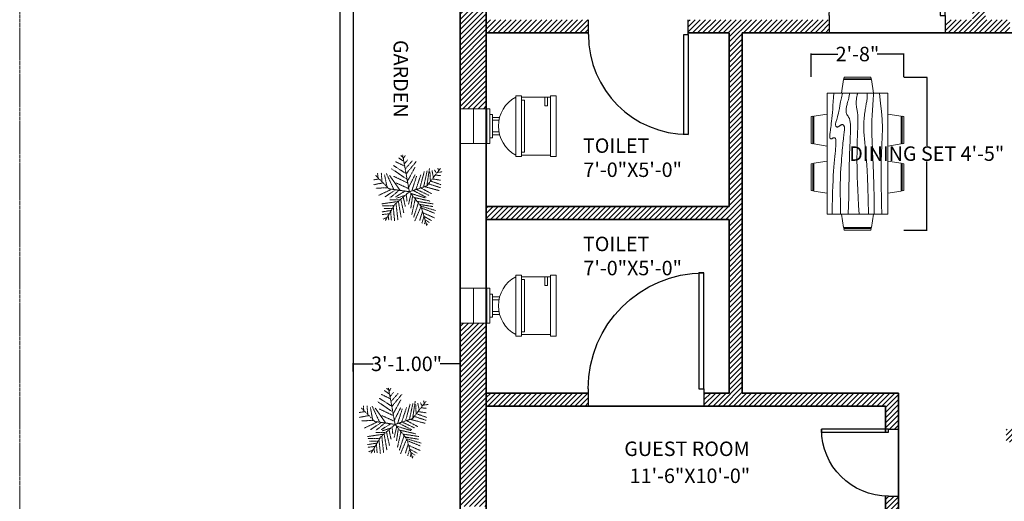
# Model space of a CAD drawing. Units: inches. Extents: x 2202345 to 2203065, y -970921 to -970107.
# Tile 3 of 5: x 2202345 to 2202685, y -970515 to -970348. Entities that reach past the tile are written whole.
import ezdxf

# ---------------------------------------------------------------- set-up
doc = ezdxf.new("R2010")
doc.units = ezdxf.units.IN
doc.header["$MEASUREMENT"] = 0
doc.linetypes.add('HIDDEN', pattern=[0.375, 0.25, -0.125])
doc.layers.get('0').update_dxf_attribs({"color": 13})
for name, color, linetype, lineweight in [('A-ANNO-DIMS', 2, 'Continuous', 18), ('A-ANNO-TTLB', 7, 'HIDDEN', 18), ('A-AREA-IDEN', 7, 'Continuous', 18), ('A-WALL-PATT', 8, 'Continuous', 13), ('C-PROP', 7, 'Continuous', 25), ('doors', 252, 'Continuous', 25), ('furniture', 250, 'Continuous', 18), ('garden', 114, 'HIDDEN', 13), ('PLUMBING FIXTURES', 8, 'Continuous', 18), ('walls', 252, 'Continuous', 35), ('windows', 173, 'Continuous', 18)]:
    doc.layers.add(name, color=color, linetype=linetype, lineweight=lineweight)
doc.styles.get("Standard").update_dxf_attribs({"font": 'arial.ttf'})
doc.dimstyles.get("Standard").update_dxf_attribs({"dimtxt": 5, "dimasz": 0.18, "dimexe": 0.18, "dimexo": 0.0625, "dimgap": 0.09, "dimtad": 0, "dimtih": 1, "dimtoh": 1, "dimzin": 0, "dimdsep": 46, "dimlunit": 3, "dimtxsty": 'Standard', "dimcen": 0.09, "dimadec": 0, "dimazin": 0, "dimtfac": 1, "dimtofl": 0, "dimtmove": 0, "dimatfit": 3, "dimfxl": 1, "dimtolj": 1, "dimtzin": 0, "dimarcsym": 0})
pattern_1 = [(45, (0, 0), (-0.8838834765, 0.8838834765), [])]

# ---------------------------------------------------------------- blocks, each defined once
blk = doc.blocks.new('Dining Set - 36 x 72 in.')
for p, q in [((-22.2343, 26.00059), (-23.4847, 17.99762)), ((-22.2304, 26), (-5.7608, 26)), ((-22, 27.5), (-22.1562, 26.50042)), ((-5.8416, 26.5), (-22.1534, 26.5)), ((-22, 27.5), (-6, 27.5)), ((-5.8437, 26.49966), (-6, 27.5)), ((-4.5152, 17.99762), (-5.7655, 25.99926)), ((5.7657, 26.00059), (4.5153, 17.99762)), ((5.7696, 26), (22.2392, 26)), ((6, 27.5), (5.8438, 26.50042)), ((22.1584, 26.5), (5.8466, 26.5)), ((6, 27.5), (22, 27.5)), ((22.1563, 26.49966), (22, 27.5)), ((23.4848, 17.99762), (22.2345, 25.99926)), ((36, 18), (-36, 18)), ((-36, 18), (-36, -18)), ((36, -18), (36, 18)), ((-45.5, 8), (-44.5004, 8.15617)), ((-45.5, 8), (-45.5, -8)), ((-44.5, -8.15843), (-44.5, 8.15338)), ((-44.0006, 8.23428), (-35.9976, 9.48474)), ((-44, 8.23041), (-44, -8.23915)), ((44.0006, 8.23428), (35.9976, 9.48474)), ((44, 8.23041), (44, -8.23915)), ((44.5, -8.15843), (44.5, 8.15338)), ((45.5, 8), (44.5005, 8.15617)), ((45.5, 8), (45.5, -8)), ((-44.4997, -8.15631), (-45.5, -8)), ((-35.9976, -9.48476), (-43.9993, -8.2345)), ((35.9976, -9.48476), (43.9993, -8.2345)), ((44.4997, -8.15631), (45.5, -8)), ((-36, -18), (36, -18)), ((-22.2343, -26.0006), (-23.4847, -17.99762)), ((-4.5152, -17.99762), (-5.7655, -25.99928)), ((5.7657, -26.0006), (4.5153, -17.99762)), ((23.4848, -17.99762), (22.2345, -25.99928)), ((-22.2304, -26), (-5.7608, -26)), ((-22, -27.5), (-22.1562, -26.50044)), ((-5.8416, -26.5), (-22.1534, -26.5)), ((-22, -27.5), (-6, -27.5)), ((-5.8437, -26.49967), (-6, -27.5)), ((5.7696, -26), (22.2392, -26)), ((6, -27.5), (5.8438, -26.50044)), ((22.1584, -26.5), (5.8466, -26.5)), ((6, -27.5), (22, -27.5)), ((22.1563, -26.49967), (22, -27.5))]:
    blk.add_line(p, q)
for points in [[(-36, 15), (-31.1772, 14.97754), (-26.8079, 14.91406), (-22.8538, 14.81543), (-19.276, 14.6875), (-16.0362, 14.53613), (-13.0957, 14.36718), (-10.4159, 14.18652), (-7.9583, 14), (-5.6904, 13.81315), (-3.6035, 13.63021), (-1.6954, 13.45508), (0.0365, 13.29166), (1.5945, 13.14388), (2.9811, 13.01562), (4.1988, 12.9108), (5.25, 12.83333), (6.1393, 12.78613), (6.8802, 12.76823), (7.4883, 12.77767), (7.9792, 12.8125), (8.3685, 12.87077), (8.6719, 12.95052), (8.9049, 13.0498), (9.0833, 13.16666), (9.2205, 13.29899), (9.3216, 13.44401), (9.3895, 13.59879), (9.4271, 13.76041), (9.4373, 13.92594), (9.4232, 14.09245), (9.3875, 14.257), (9.3333, 14.41666), (9.2638, 14.56917), (9.1836, 14.71484), (9.0975, 14.85465), (9.0104, 14.98958), (8.9272, 15.1206), (8.8529, 15.2487), (8.7922, 15.37483), (8.75, 15.5), (8.7305, 15.62467), (8.7344, 15.74739), (8.7617, 15.86621), (8.8125, 15.97916), (8.8867, 16.08431), (8.9844, 16.17968), (9.1055, 16.26334), (9.25, 16.33333), (9.4189, 16.38802), (9.6172, 16.42708), (9.8506, 16.45052), (10.125, 16.45833), (10.4463, 16.45052), (10.8203, 16.42708), (11.2529, 16.38802), (11.75, 16.33333), (12.3184, 16.26318), (12.9694, 16.17838), (13.7151, 16.07991), (14.5677, 15.96875), (15.5395, 15.84586), (16.6426, 15.71224), (17.8893, 15.56884), (19.2917, 15.41666), (20.859, 15.25667), (22.5879, 15.08984), (24.4721, 14.91715), (26.5052, 14.73958), (28.6809, 14.5581), (30.9929, 14.3737), (33.4347, 14.18733), (36, 14)], [(-36, 10), (-28.9766, 10.14274), (-23.1725, 10.20442), (-18.4241, 10.19775), (-14.5677, 10.13541), (-11.4399, 10.03011), (-8.877, 9.89453), (-6.7154, 9.74137), (-4.7917, 9.58333), (-2.9698, 9.43082), (-1.2246, 9.28515), (0.4415, 9.14534), (2.026, 9.01041), (3.5266, 8.87939), (4.9408, 8.7513), (6.266, 8.62516), (7.5, 8.5), (8.6411, 8.37549), (9.6914, 8.2539), (10.6538, 8.13818), (11.5312, 8.03125), (12.3267, 7.93603), (13.043, 7.85547), (13.6831, 7.79248), (14.25, 7.75), (14.7471, 7.7303), (15.1797, 7.73307), (15.5537, 7.75732), (15.875, 7.80208), (16.1494, 7.86637), (16.3828, 7.94922), (16.5811, 8.04964), (16.75, 8.16666), (16.8944, 8.29915), (17.0143, 8.44531), (17.1089, 8.60319), (17.1771, 8.77083), (17.218, 8.94629), (17.2305, 9.1276), (17.2137, 9.31282), (17.1667, 9.5), (17.0895, 9.6875), (16.987, 9.875), (16.8649, 10.0625), (16.7292, 10.25), (16.5856, 10.4375), (16.4401, 10.625), (16.2985, 10.8125), (16.1667, 11), (16.05, 11.18733), (15.9518, 11.3737), (15.8752, 11.5581), (15.8229, 11.73958), (15.798, 11.91715), (15.8034, 12.08984), (15.842, 12.25667), (15.9167, 12.41666), (16.0295, 12.56836), (16.1784, 12.70833), (16.3605, 12.83268), (16.5729, 12.9375), (16.8127, 13.01888), (17.0768, 13.07291), (17.3625, 13.0957), (17.6667, 13.08333), (17.9894, 13.03312), (18.3418, 12.94726), (18.7382, 12.82918), (19.1927, 12.68229), (19.7195, 12.51001), (20.3327, 12.31575), (21.0465, 12.10294), (21.875, 11.875), (22.8357, 11.63354), (23.959, 11.37304), (25.2786, 11.08618), (26.8282, 10.76562), (28.6414, 10.40405), (30.752, 9.99414), (33.1936, 9.52856), (36, 9)], [(-36, 5.5), (-30.7157, 5.3348), (-26.069, 5.20963), (-21.9946, 5.11767), (-18.4271, 5.05208), (-15.3009, 5.00602), (-12.5508, 4.97265), (-10.1112, 4.94515), (-7.9167, 4.91666), (-5.909, 4.88167), (-4.0586, 4.83984), (-2.3429, 4.79215), (-0.7396, 4.73958), (0.7739, 4.6831), (2.22, 4.6237), (3.6213, 4.56233), (5, 4.5), (6.373, 4.43782), (7.7344, 4.3776), (9.0723, 4.32129), (10.375, 4.27083), (11.6309, 4.22819), (12.8281, 4.19531), (13.9551, 4.17415), (15, 4.16666), (15.954, 4.17448), (16.819, 4.19791), (17.6001, 4.23698), (18.3021, 4.29166), (18.9299, 4.36198), (19.4883, 4.44791), (19.9823, 4.54948), (20.4167, 4.66666), (20.7969, 4.79899), (21.1302, 4.94401), (21.4245, 5.09879), (21.6875, 5.26041), (21.9271, 5.42594), (22.1511, 5.59245), (22.3672, 5.757), (22.5834, 5.91666), (22.8065, 6.06868), (23.0404, 6.21093), (23.2879, 6.34147), (23.5521, 6.45833), (23.8358, 6.55957), (24.142, 6.64323), (24.4735, 6.70735), (24.8334, 6.75), (25.2235, 6.76969), (25.642, 6.76692), (26.0858, 6.74267), (26.5521, 6.69791), (27.0379, 6.63362), (27.5404, 6.55078), (28.0565, 6.45036), (28.5834, 6.33333), (29.1242, 6.19987), (29.7071, 6.04687), (30.3661, 5.87044), (31.1354, 5.66666), (32.0493, 5.43164), (33.142, 5.16146), (34.4475, 4.85221), (36, 4.5)], [(-36, -1), (-30.7915, -0.6591), (-26.0195, -0.38216), (-21.6519, -0.16284), (-17.6563, 0.00521), (-14.0005, 0.12833), (-10.6523, 0.21289), (-7.5796, 0.26522), (-4.75, 0.29166), (-2.134, 0.29793), (0.2878, 0.28711), (2.5317, 0.26163), (4.6146, 0.22396), (6.5529, 0.17651), (8.3633, 0.12174), (10.0623, 0.06209), (11.6667, 0), (13.1899, -0.06201), (14.6341, -0.1211), (15.9982, -0.17432), (17.2813, -0.21875), (18.4823, -0.25147), (19.6003, -0.26953), (20.6343, -0.27002), (21.5834, -0.25), (22.4481, -0.20768), (23.2357, -0.14584), (23.9549, -0.06836), (24.6146, 0.02083), (25.2235, 0.11784), (25.7904, 0.21875), (26.3241, 0.31966), (26.8334, 0.41666), (27.3265, 0.50618), (27.8099, 0.58593), (28.2894, 0.65397), (28.7709, 0.70833), (29.2601, 0.74707), (29.763, 0.76823), (30.2855, 0.76985), (30.8334, 0.75), (31.4088, 0.70784), (31.9994, 0.64713), (32.589, 0.57275), (33.1615, 0.48958), (33.7008, 0.4025), (34.1908, 0.3164), (34.6153, 0.23616), (34.9584, 0.16666), (35.2099, 0.11165), (35.3848, 0.07031), (35.504, 0.04069), (35.5886, 0.02083), (35.6594, 0.00879), (35.7377, 0.0026), (35.8442, 0.00032), (36, 0)], [(-36, -6.5), (-27.1843, -6.31267), (-20.084, -6.1263), (-14.469, -5.9419), (-10.1094, -5.76042), (-6.7752, -5.58285), (-4.2363, -5.41016), (-2.2629, -5.24333), (-0.625, -5.08334), (0.8708, -4.93099), (2.2715, -4.78646), (3.5872, -4.64974), (4.8281, -4.52084), (6.0046, -4.39974), (7.127, -4.28646), (8.2053, -4.18099), (9.25, -4.08334), (10.2705, -3.99382), (11.2734, -3.91407), (12.2647, -3.84603), (13.25, -3.79167), (14.2354, -3.75293), (15.2266, -3.73177), (16.2295, -3.73015), (17.25, -3.75), (18.2912, -3.79248), (19.3451, -3.85547), (20.4009, -3.93604), (21.4479, -4.03125), (22.4754, -4.13819), (23.4727, -4.25391), (24.4289, -4.37549), (25.3334, -4.5), (26.1785, -4.62492), (26.9694, -4.74935), (27.7145, -4.87281), (28.4219, -4.99479), (29.1, -5.11483), (29.7572, -5.23242), (30.4016, -5.34709), (31.0417, -5.45834), (31.6837, -5.56437), (32.3262, -5.65821), (32.9658, -5.73153), (33.599, -5.77604), (34.2224, -5.78345), (34.8327, -5.74545), (35.4264, -5.65373), (36, -5.5)], [(-36, -10), (-26.4022, -9.81299), (-18.4675, -9.62891), (-11.9839, -9.45069), (-6.7396, -9.28125), (-2.5226, -9.12354), (0.8789, -8.98047), (3.6769, -8.85498), (6.0833, -8.75), (8.2767, -8.66765), (10.3021, -8.60677), (12.1712, -8.56543), (13.8958, -8.54167), (15.4876, -8.53353), (16.9583, -8.53907), (18.3197, -8.55632), (19.5834, -8.58334), (20.7616, -8.61841), (21.8685, -8.66081), (22.9188, -8.71004), (23.9271, -8.76563), (24.9081, -8.82707), (25.8763, -8.89388), (26.8465, -8.96558), (27.8334, -9.04167), (28.8474, -9.12118), (29.8828, -9.20117), (30.93, -9.27824), (31.9792, -9.34896), (33.0205, -9.40991), (34.0443, -9.45768), (35.0407, -9.48885), (36, -9.5)], [(-36, -14.5), (-30.0881, -14.33513), (-25.0332, -14.21224), (-20.7312, -14.12647), (-17.0781, -14.07292), (-13.97, -14.04671), (-11.3027, -14.04297), (-8.9724, -14.05681), (-6.875, -14.08334), (-4.9224, -14.11833), (-3.0905, -14.16016), (-1.3709, -14.20785), (0.2448, -14.26042), (1.7647, -14.3169), (3.1973, -14.3763), (4.5507, -14.43767), (5.8333, -14.5), (7.0554, -14.5621), (8.235, -14.62175), (9.3922, -14.67652), (10.5469, -14.72396), (11.7192, -14.76164), (12.929, -14.78711), (14.1965, -14.79794), (15.5417, -14.79167), (16.9933, -14.76424), (18.6152, -14.70508), (20.4804, -14.60197), (22.6615, -14.44271), (25.2312, -14.21509), (28.2624, -13.9069), (31.8277, -13.50594), (36, -13)]]:
    blk.add_lwpolyline(points)
blk = doc.blocks.new('*U2')
for p, q in [((-10, 22), (-10, 12)), ((-10, 21), (-7, 21)), ((-7, 21), (-7, 20)), ((10, 12), (10, 22)), ((-7, 20), (-10, 20)), ((10.5, 12), (-10.5, 12)), ((-10.5, 10), (-10.5, 12)), ((9, 13), (-9, 13)), ((-9, 13), (-9, 12)), ((9, 12), (9, 13)), ((10.5, 12), (10.5, 10)), ((10.5, 10), (-10.5, 10)), ((-3, 4.4065), (-3, 2)), ((-2, 2), (-2, 4.1658)), ((2, 4.1658), (2, 2)), ((3, 2), (3, 4.4065)), ((4, 2), (-4, 2)), ((-4, 2), (-4, 1)), ((4, 1), (4, 2))]:
    blk.add_line(p, q)
for points in [[(10.5, 22), (10.5, 24), (-10.5, 24), (-10.5, 22)], [(6, 0), (6, 1), (-6, 1), (-6, 0)]]:
    blk.add_lwpolyline(points, close=True)
blk.add_arc((0, 15.3333), 11.3333, 208.0725, 331.9275)
blk = doc.blocks.new('*U12')
for p, q in [((0, 0), (0, -6)), ((40, 0), (40, -6))]:
    blk.add_line(p, q)
blk.add_lwpolyline([(0, 0), (0, 40), (1.75, 40), (1.75, 0)], close=True)
blk.add_arc((0, 0), 40, 0, 90)
blk = doc.blocks.new('*D14')
at = {"layer": 'A-ANNO-DIMS', "color": 0, "lineweight": -2, "transparency": 16777216}
for p, q in [((2202459.68, -970469.7), (2202459.68, -970466.84)), ((2202459.86, -970467.02), (2202466.59, -970467.02)), ((2202496.5, -970467.02), (2202489.77, -970467.02)), ((2202496.68, -970469.7), (2202496.68, -970466.84))]:
    blk.add_line(p, q, dxfattribs=at)
at = {"layer": 'A-ANNO-DIMS', "color": 0, "transparency": 16777216}
for points in [[(2202459.86, -970466.99), (2202459.86, -970467.05), (2202459.68, -970467.02)], [(2202496.5, -970466.99), (2202496.5, -970467.05), (2202496.68, -970467.02)]]:
    blk.add_solid(points, dxfattribs=at)
at = {"layer": 'Defpoints', "color": 0, "transparency": 16777216}
for p in [(2202496.68, -970467.02), (2202459.68, -970469.77), (2202496.68, -970469.77)]:
    blk.add_point(p, dxfattribs=at)
at = {"layer": 'A-ANNO-DIMS', "color": 0, "transparency": 16777216, "insert": (2202478.18, -970467.02), "char_height": 5, "attachment_point": 5}
blk.add_mtext('\\A1;3\'-1.00"', dxfattribs=at)
blk = doc.blocks.new('*U23')
for p, q in [((-7.288, 39.707), (-21.778, 46.673)), ((-8.737, 47.138), (-17.069, 52.711)), ((-10.186, 53.64), (-13.084, 55.962)), ((0, 0), (-10.5, 57)), ((-9.099, 51.782), (-6.563, 55.962)), ((-7.65, 43.423), (-2.578, 49.46)), ((-5.839, 35.992), (4.667, 48.067)), ((-5.114, 27.632), (10.463, 46.673)), ((-3.665, 19.273), (-27.574, 35.527)), ((-5.114, 28.097), (-24.676, 40.636)), ((-2.941, 16.486), (8.652, 37.85)), ((16.259, 5.805), (23.142, 31.348)), ((22.055, 7.198), (27.489, 32.277)), ((27, 9), (48, 36)), ((27.127, 9.056), (31.112, 35.992)), ((31.836, 30.883), (32.561, 16.486)), ((35.096, 32.741), (37.27, 22.524)), ((38.719, 34.134), (41.979, 28.561)), ((43.791, 29.954), (51.036, 30.883)), ((44.153, 36.456), (45.239, 32.741)), ((-47.498, 19.737), (-55.83, 18.344)), ((-31.5, 4.5), (-52.5, 25.5)), ((-48.585, 21.131), (-49.309, 29.026)), ((-43.513, 28.561), (-42.427, 15.558)), ((-38.442, 26.239), (-34.819, 7.663)), ((-35.544, 28.097), (-24.314, 3.947)), ((-14.533, 2.09), (-30.834, 25.31)), ((-24.314, 23.917), (-2.941, 13.7)), ((-1.129, 6.734), (9.014, 26.704)), ((3.942, 1.625), (11.187, 24.381)), ((10.101, 3.483), (17.708, 26.239)), ((33.285, 16.486), (48.862, 10.913)), ((36.183, 19.737), (48.137, 17.88)), ((40.53, 25.775), (48.862, 24.846)), ((-40.615, 13.7), (-55.105, 10.913)), ((-33.37, 6.269), (-52.207, 5.34)), ((-28.299, 3.483), (-47.86, -5.805)), ((-21.416, 3.018), (-38.079, -8.128)), ((0, 0), (-31.5, 4.5)), ((-15.982, 2.09), (-30.11, -9.521)), ((0, 0), (-22.5, -19.5)), ((-6.563, 1.161), (-21.416, -8.128)), ((-20.691, 13.7), (-1.129, 4.876)), ((0, 0), (27, 9)), ((0, 0), (18, -22.5)), ((6.478, 1.625), (26.04, -8.592)), ((11.187, 3.483), (30.749, -5.805)), ((18.07, 5.805), (35.096, -3.483)), ((24.229, 7.663), (46.688, 1.625)), ((29.662, 12.307), (48.137, 6.269)), ((-17.431, -15.094), (-42.789, -18.809)), ((-15.257, -12.772), (-30.11, -12.772)), ((-6.563, -5.805), (-19.967, -9.985)), ((-17.069, -15.094), (-12.721, -40.172)), ((-13.446, -11.378), (-8.737, -32.741)), ((-9.461, -8.592), (-6.201, -23.453)), ((-4.752, -3.483), (-3.665, -14.629)), ((2.493, -3.019), (-1.491, -20.202)), ((1.769, -2.555), (24.229, -9.521)), ((5.029, -6.27), (2.131, -25.775)), ((9.014, -11.378), (3.58, -35.992)), ((7.565, -9.056), (32.198, -14.629)), ((12.274, -15.094), (36.907, -18.809)), ((-28.299, -29.026), (-42.789, -31.348)), ((-24.314, -21.596), (-42.427, -22.06)), ((-26.849, -26.24), (-40.253, -25.775)), ((-22.5, -19.5), (-37.5, -45)), ((-25.038, -23.918), (-22.865, -45.281)), ((-20.691, -18.345), (-17.793, -44.352)), ((14.085, -16.951), (6.478, -40.172)), ((18.07, -22.524), (8.289, -45.745)), ((20.244, -30.419), (15.897, -44.816)), ((16.259, -19.738), (36.183, -22.989)), ((18, -22.5), (27, -52.5)), ((18.433, -22.524), (40.53, -29.026)), ((19.157, -25.311), (38.719, -33.206)), ((-30.834, -34.135), (-42.427, -35.528)), ((-34.457, -39.708), (-40.978, -42.494)), ((-32.646, -36.921), (-31.921, -44.352)), ((-29.023, -30.884), (-27.936, -43.887)), ((22.78, -37.85), (19.519, -48.532)), ((21.331, -32.741), (39.081, -40.636)), ((22.78, -38.314), (34.372, -44.816)), ((24.591, -45.745), (23.142, -50.854)), ((24.591, -43.423), (30.749, -47.603)), ((26.764, -49.925), (28.213, -50.854))]:
    blk.add_line(p, q)
blk = doc.blocks.new('*D35')
at = {"layer": 'A-ANNO-DIMS', "color": 0, "lineweight": -2, "transparency": 16777216}
for p, q in [((2202650.03, -970367.92), (2202658.08, -970367.92)), ((2202657.9, -970368.1), (2202657.9, -970391.7)), ((2202657.9, -970420.66), (2202657.9, -970397.05)), ((2202650.03, -970420.84), (2202658.08, -970420.84))]:
    blk.add_line(p, q, dxfattribs=at)
at = {"layer": 'A-ANNO-DIMS', "color": 0, "transparency": 16777216}
for points in [[(2202657.87, -970368.1), (2202657.93, -970368.1), (2202657.9, -970367.92)], [(2202657.87, -970420.66), (2202657.93, -970420.66), (2202657.9, -970420.84)]]:
    blk.add_solid(points, dxfattribs=at)
at = {"layer": 'Defpoints', "color": 0, "transparency": 16777216}
for p in [(2202649.96, -970367.92), (2202657.9, -970367.92), (2202649.96, -970420.84)]:
    blk.add_point(p, dxfattribs=at)
at = {"layer": 'A-ANNO-DIMS', "color": 0, "transparency": 16777216, "insert": (2202657.9, -970394.38), "char_height": 5, "attachment_point": 5}
blk.add_mtext('\\A1;DINING SET 4\'-5"', dxfattribs=at)
blk = doc.blocks.new('*D36')
at = {"layer": 'A-ANNO-DIMS', "color": 0, "lineweight": -2, "transparency": 16777216}
for p, q in [((2202617.98, -970367.86), (2202617.98, -970359.8)), ((2202618.16, -970359.98), (2202627.19, -970359.98)), ((2202649.78, -970359.98), (2202640.75, -970359.98)), ((2202649.96, -970367.86), (2202649.96, -970359.8))]:
    blk.add_line(p, q, dxfattribs=at)
at = {"layer": 'A-ANNO-DIMS', "color": 0, "transparency": 16777216}
for points in [[(2202618.16, -970359.95), (2202618.16, -970360.01), (2202617.98, -970359.98)], [(2202649.78, -970359.95), (2202649.78, -970360.01), (2202649.96, -970359.98)]]:
    blk.add_solid(points, dxfattribs=at)
at = {"layer": 'Defpoints', "color": 0, "transparency": 16777216}
for p in [(2202617.98, -970359.98), (2202617.98, -970367.92), (2202649.96, -970367.92)]:
    blk.add_point(p, dxfattribs=at)
at = {"layer": 'A-ANNO-DIMS', "color": 0, "transparency": 16777216, "insert": (2202633.97, -970359.98), "char_height": 5, "attachment_point": 5}
blk.add_mtext('\\A1;2\'-8"', dxfattribs=at)

msp = doc.modelspace()

# ---------------------------------------------------------------- hatches: boundary and pattern name
at = {"layer": 'A-WALL-PATT'}
h = msp.add_hatch(dxfattribs=at)
h.set_pattern_fill('ANSI31', color=256, scale=10)
h.set_pattern_definition(pattern_1)
h.paths.add_polyline_path([(2202648.182, -970512.768), (2202644.707, -970512.768, -0.0110733), (2202643.682, -970512.746), (2202643.682, -970601.606), (2202609.913, -970601.606), (2202609.913, -970610.606), (2202643.682, -970610.606), (2202643.682, -970619.168), (2202647.677, -970619.168, -0.0047326), (2202648.182, -970619.173)])
h.paths.add_polyline_path([(2202643.682, -970610.606), (2202636.037, -970610.606), (2202636.037, -970659.106), (2202643.682, -970659.106)])
h.paths.add_polyline_path([(2202722.39, -970654.606), (2202722.39, -970650.106), (2202648.182, -970650.106), (2202648.182, -970645.806), (2202647.677, -970645.806), (2202643.682, -970645.806), (2202643.682, -970659.106), (2202722.39, -970659.106)])
h.paths.add_polyline_path([(2202846.182, -970650.106), (2202798.148, -970650.106), (2202798.148, -970659.106), (2202846.182, -970659.106)])
h.paths.add_polyline_path([(2202855.182, -970619.995), (2202846.182, -970619.995), (2202846.182, -970682.124), (2202855.182, -970682.124)])
h.paths.add_polyline_path([(2202855.182, -970434.646), (2202846.182, -970434.646), (2202846.182, -970545.038), (2202855.182, -970545.038)])
h.paths.add_polyline_path([(2202903.182, -970745.106), (2202855.182, -970745.106), (2202855.182, -970729.208), (2202846.182, -970729.208), (2202846.182, -970745.106), (2202725.91, -970745.106), (2202725.91, -970754.106), (2202903.182, -970754.106)])
h.paths.add_polyline_path([(2202846.182, -970489.606), (2202767.486, -970489.606, -0.1570508), (2202766.685, -970489.864), (2202739.229, -970489.864, -0.1570508), (2202738.428, -970489.606), (2202685.343, -970489.606), (2202685.343, -970494.106), (2202846.182, -970494.106)])
h.paths.add_polyline_path([(2202648.182, -970477.106), (2202594.182, -970477.106), (2202594.182, -970352.606), (2202624.243, -970352.606), (2202624.243, -970348.106), (2202575.482, -970348.106), (2202575.482, -970352.606), (2202589.682, -970352.606), (2202589.682, -970412.606), (2202505.682, -970412.606), (2202505.682, -970417.106), (2202589.682, -970417.106), (2202589.682, -970477.106), (2202580.925, -970477.106), (2202580.925, -970481.606), (2202643.682, -970481.606), (2202643.682, -970489.606), (2202644.707, -970489.606), (2202648.182, -970489.606)])
h.paths.add_polyline_path([(2202505.682, -970305.515), (2202496.682, -970305.515), (2202496.682, -970378.877), (2202501.298, -970378.877), (2202505.682, -970378.877)])
h.paths.add_polyline_path([(2202540.998, -970348.106), (2202505.682, -970348.106), (2202505.682, -970352.606), (2202540.998, -970352.606)], flags=17)
h.paths.add_polyline_path([(2202505.682, -970452.918), (2202496.682, -970452.918), (2202496.682, -970516.267), (2202505.682, -970516.267)])
h.paths.add_polyline_path([(2202505.682, -970210.106), (2202898.682, -970210.106), (2202898.682, -970294.106), (2202889.459, -970294.106), (2202889.459, -970303.106), (2202907.682, -970303.106), (2202907.682, -970201.106), (2202496.682, -970201.106), (2202496.682, -970242.728), (2202505.682, -970242.728)])
h.paths.add_polyline_path([(2202678.182, -970210.106), (2202673.682, -970210.106), (2202673.682, -970348.106), (2202664.243, -970348.106), (2202664.243, -970352.606), (2202686.569, -970352.606), (2202686.569, -970348.106), (2202678.182, -970348.106)])
h.paths.add_polyline_path([(2202752.572, -970321.843), (2202794.204, -970321.843), (2202794.204, -970314.185), (2202752.572, -970314.185)], flags=9)
h.paths.add_polyline_path([(2202750.562, -970312.127), (2202793.125, -970312.127), (2202793.125, -970304.366), (2202750.562, -970304.366)], flags=9)
h = msp.add_hatch(dxfattribs=at)
h.set_pattern_fill('ANSI31', color=256, scale=10)
h.set_pattern_definition(pattern_1)
h.paths.add_polyline_path([(2202540.925, -970477.106), (2202505.682, -970477.106), (2202505.682, -970481.606), (2202540.925, -970481.606)])
h.paths.add_polyline_path([(2202553.677, -970601.606), (2202505.682, -970601.606), (2202505.682, -970565.796), (2202496.682, -970565.796), (2202496.682, -970610.606), (2202553.677, -970610.606), (2202553.677, -970606.106)])

# ---------------------------------------------------------------- linework, layer by layer
at = {"layer": 'A-ANNO-TTLB'}
msp.add_line((2202344.52, -970106.63), (2202344.52, -970920.555), dxfattribs=at)
at = {"layer": 'C-PROP'}
for p, q in [((2202455.182, -970201.106), (2202455.182, -970804.606)), ((2202459.682, -970205.606), (2202459.682, -970800.106))]:
    msp.add_line(p, q, dxfattribs=at)
at = {"layer": 'walls'}
for p, q in [((2202496.682, -970201.106), (2202496.682, -970610.606)), ((2202505.682, -970210.106), (2202505.682, -970601.606)), ((2202505.682, -970352.606), (2202540.998, -970352.606)), ((2202575.482, -970352.606), (2202589.682, -970352.606)), ((2202589.682, -970352.606), (2202589.682, -970412.606)), ((2202594.182, -970352.606), (2202594.182, -970477.106)), ((2202594.182, -970352.606), (2202846.182, -970352.606)), ((2202505.682, -970412.606), (2202589.682, -970412.606)), ((2202505.682, -970417.106), (2202589.682, -970417.106)), ((2202589.682, -970417.106), (2202589.682, -970477.106)), ((2202505.682, -970477.106), (2202540.925, -970477.106)), ((2202580.925, -970477.106), (2202589.682, -970477.106)), ((2202594.182, -970477.106), (2202648.182, -970477.106)), ((2202648.182, -970477.106), (2202648.182, -970619.173)), ((2202505.682, -970481.606), (2202643.682, -970481.606)), ((2202643.682, -970481.606), (2202643.682, -970490.619)), ((2202643.682, -970512.746), (2202643.682, -970601.606))]:
    msp.add_line(p, q, dxfattribs=at)
at = {"layer": 'windows'}
for p, q in [((2202505.915, -970378.877), (2202496.682, -970378.877)), ((2202496.682, -970378.877), (2202501.298, -970378.877)), ((2202501.298, -970378.877), (2202501.298, -970390.877)), ((2202501.298, -970390.877), (2202496.682, -970390.877)), ((2202496.682, -970390.877), (2202505.682, -970390.877)), ((2202505.915, -970440.918), (2202496.682, -970440.918)), ((2202496.682, -970440.918), (2202501.298, -970440.918)), ((2202501.298, -970440.918), (2202501.298, -970452.918)), ((2202505.682, -970452.918), (2202496.682, -970452.918)), ((2202501.298, -970452.918), (2202505.682, -970452.918))]:
    msp.add_line(p, q, dxfattribs=at)

# ---------------------------------------------------------------- block references
at = {"layer": 'doors', "xscale": -1}
for p in [(2202664.243, -970346.606), (2202580.925, -970475.606)]:
    msp.add_blockref('*U12', p, dxfattribs=at)
at = {"layer": 'doors'}
for p, xscale, yscale, zscale, rotation in [((2202575.482, -970353.278), 0.8621024727113805, 0.8621024727113805, 0.8621024727113805, 180), ((2202644.707, -970489.606), -0.5790702303642968, 0.5790702303642968, 0.5790702303642968, 90)]:
    msp.add_blockref('*U12', p, dxfattribs=dict(at, xscale=xscale, yscale=yscale, zscale=zscale, rotation=rotation))
at = {"layer": 'furniture', "xscale": 0.581512735032396, "yscale": 0.581512735032396, "zscale": 0.581512735032396, "rotation": 90}
msp.add_blockref('Dining Set - 36 x 72 in.', (2202633.972, -970394.378), dxfattribs=at)
at = {"layer": 'garden', "xscale": 0.2228486455557245, "yscale": 0.2228486455557245, "zscale": 0.2228486455557245}
for p in [(2202479.157, -970407.547), (2202474.232, -970487.941)]:
    msp.add_blockref('*U23', p, dxfattribs=at)
at = {"layer": 'PLUMBING FIXTURES', "rotation": 270}
for p in [(2202505.915, -970384.877), (2202505.915, -970446.918)]:
    msp.add_blockref('*U2', p, dxfattribs=at)

# ---------------------------------------------------------------- texts
at = {"layer": 'A-AREA-IDEN'}
msp.add_text('GARDEN', height=5, rotation=270, dxfattribs=at).set_placement((2202473.697, -970355.127))
for s, p in [('TOILET', (2202539.115, -970394.122)), ('7\'-0"X5\'-0"', (2202539.289, -970402.453)), ('TOILET', (2202539.115, -970428.087)), ('7\'-0"X5\'-0"', (2202539.289, -970436.418)), ('GUEST ROOM', (2202553.401, -970498.867)), ('11\'-6"X10\'-0"', (2202555.27, -970508.2))]:
    msp.add_text(s, height=5, dxfattribs=at).set_placement(p)

# ---------------------------------------------------------------- dimensions: what is measured, and where the dimension line sits
at = {"layer": 'A-ANNO-DIMS'}
dim = msp.add_linear_dim(base=(2202617.981, -970359.981), p1=(2202649.964, -970367.919), p2=(2202617.981, -970367.919), angle=180, dimstyle='Standard', override={"dimdec": 1, "dimlfac": 1, "dimrnd": 0, "dimzin": 1, "dimdsep": 46, "dimlunit": 4, "dimfrac": 2}, dxfattribs=at)
dim.commit()
dim.dimension.update_dxf_attribs({"geometry": '*D36', "text_midpoint": (2202633.972, -970359.981)})
dim = msp.add_linear_dim(base=(2202657.902, -970367.919), p1=(2202649.964, -970420.837), p2=(2202649.964, -970367.919), angle=90, text='DINING SET <>', dimstyle='Standard', override={"dimdec": 1, "dimlfac": 1, "dimrnd": 0, "dimzin": 1, "dimdsep": 46, "dimlunit": 4, "dimfrac": 2}, dxfattribs=at)
dim.commit()
dim.dimension.update_dxf_attribs({"geometry": '*D35', "text_midpoint": (2202657.902, -970394.378)})
dim = msp.add_linear_dim(base=(2202496.682, -970467.02), p1=(2202459.682, -970469.767), p2=(2202496.682, -970469.767), dimstyle='Standard', override={"dimclrd": 0, "dimclre": 0, "dimclrt": 0}, dxfattribs=at)
dim.commit()
dim.dimension.update_dxf_attribs({"geometry": '*D14', "text_midpoint": (2202478.182, -970467.02)})

doc.saveas('drawing.dxf')
